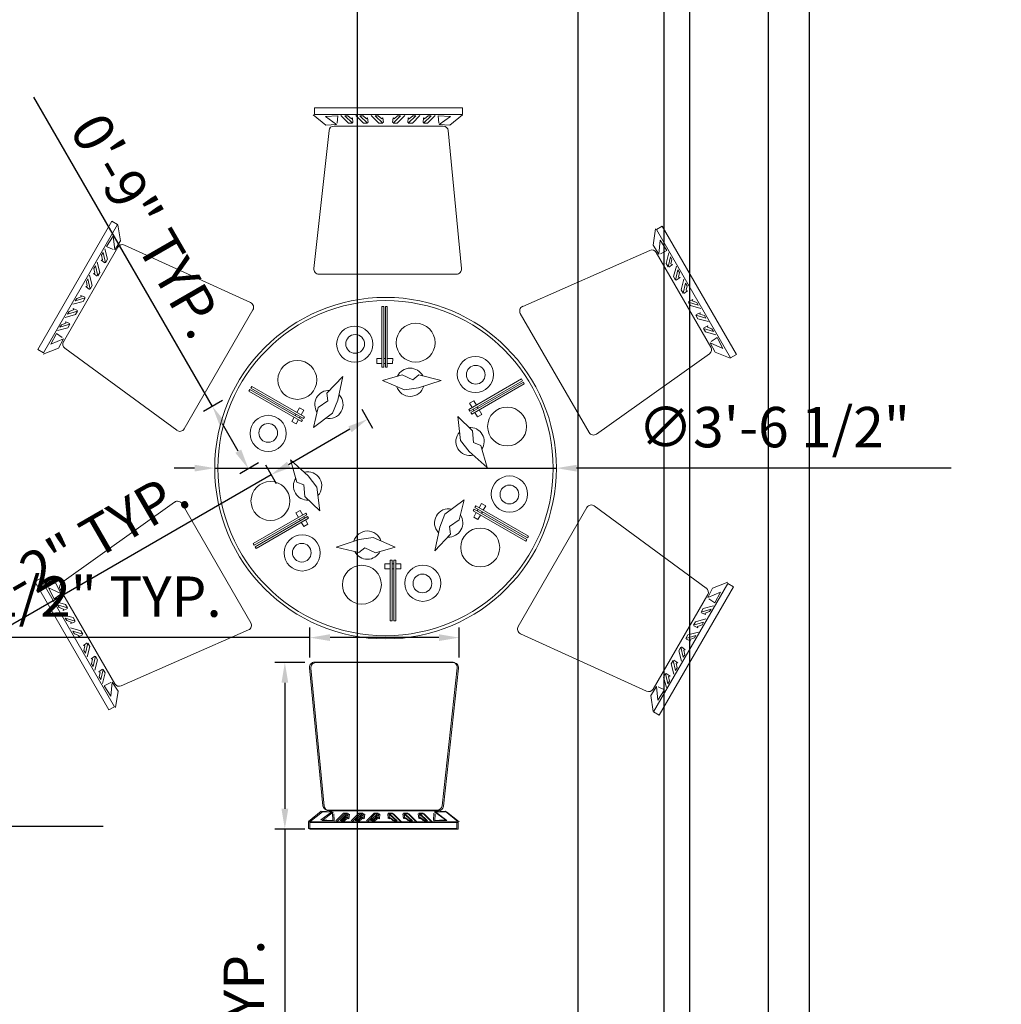
# Model space of a CAD drawing. Units: inches. Extents: x 2923 to 3500, y 1684 to 2381.
# Tile 8 of 12: x 3125 to 3246, y 1992 to 2114. Entities that reach past the tile are written whole.
import ezdxf

# ---------------------------------------------------------------- set-up
doc = ezdxf.new("R2010")
doc.units = ezdxf.units.IN
doc.layers.add('A-ANNO-DIMS', color=2, linetype='Continuous', lineweight=18)
doc.layers.add('Furniture', color=7, linetype='Continuous', lineweight=15)
doc.styles.get("Standard").update_dxf_attribs({"font": 'txt', "height": 5})
doc.dimstyles.new('ISO-25', dxfattribs={"dimtxt": 5, "dimasz": 2.5, "dimexe": 1.25, "dimexo": 0.625, "dimtad": 1, "dimlunit": 3, "dimtxsty": 'Standard', "dimcen": 2.5, "dimadec": 0, "dimazin": 0, "dimtfac": 1, "dimtmove": 0, "dimatfit": 3, "dimfxl": 1, "dimarcsym": 0})

# ---------------------------------------------------------------- blocks, each defined once
blk = doc.blocks.new('CHAIR-DINING')
for p, q in [((0, 19.73), (1.57, 18.47)), ((0.13, 20.61), (0.13, 19.79)), ((18.48, 20.61), (0.13, 20.61)), ((0.13, 19.79), (18.48, 19.79)), ((1.51, 19.54), (3.02, 19.6)), ((2.89, 18.53), (1.51, 19.54)), ((3.02, 19.6), (2.95, 18.72)), ((3.39, 19.66), (4.34, 18.72)), ((3.9, 19.6), (4.27, 19.6)), ((4.84, 18.72), (3.9, 19.6)), ((4.27, 19.6), (4.71, 19.22)), ((5.28, 19.66), (6.22, 18.72)), ((5.78, 19.6), (6.16, 19.6)), ((6.73, 18.72), (5.78, 19.6)), ((6.16, 19.6), (6.6, 19.22)), ((7.16, 19.66), (8.11, 18.72)), ((7.67, 19.6), (8.04, 19.6)), ((8.61, 18.72), (7.67, 19.6)), ((8.04, 19.6), (8.48, 19.22)), ((9.87, 18.72), (10.81, 19.6)), ((10.43, 19.6), (9.99, 19.22)), ((11.31, 19.66), (10.37, 18.72)), ((10.81, 19.6), (10.43, 19.6)), ((11.75, 18.72), (12.7, 19.6)), ((12.32, 19.6), (11.88, 19.22)), ((13.2, 19.66), (12.26, 18.72)), ((12.7, 19.6), (12.32, 19.6)), ((13.64, 18.72), (14.58, 19.6)), ((14.2, 19.6), (13.76, 19.22)), ((15.08, 19.66), (14.14, 18.72)), ((14.58, 19.6), (14.2, 19.6)), ((15.46, 19.6), (15.52, 18.72)), ((16.97, 19.54), (15.46, 19.6)), ((15.59, 18.53), (16.97, 19.54)), ((18.48, 19.73), (16.91, 18.47)), ((18.48, 19.79), (18.48, 20.61)), ((1.57, 18.47), (2.89, 18.53)), ((2.57, 18.34), (16.08, 18.34)), ((4.34, 18.72), (4.84, 18.72)), ((4.71, 19.22), (4.84, 19.35)), ((4.84, 19.35), (4.9, 18.78)), ((6.22, 18.72), (6.73, 18.72)), ((6.6, 19.22), (6.73, 19.35)), ((6.73, 19.35), (6.79, 18.78)), ((8.11, 18.72), (8.61, 18.72)), ((8.48, 19.22), (8.61, 19.35)), ((8.61, 19.35), (8.67, 18.78)), ((9.87, 19.35), (9.8, 18.78)), ((9.99, 19.22), (9.87, 19.35)), ((10.37, 18.72), (9.87, 18.72)), ((11.75, 19.35), (11.69, 18.78)), ((11.88, 19.22), (11.75, 19.35)), ((12.26, 18.72), (11.75, 18.72)), ((13.64, 19.35), (13.58, 18.78)), ((13.76, 19.22), (13.64, 19.35)), ((14.14, 18.72), (13.64, 18.72)), ((16.91, 18.47), (15.59, 18.53)), ((0.08, 0.7), (1.95, 17.78)), ((16.71, 17.78), (18.35, 0.69)), ((17.72, 0), (0.7, 0))]:
    blk.add_line(p, q)
for centre, start, end in [((2.57, 17.72), 90, 173.7428), ((16.08, 17.72), 5.4801, 90), ((0.7, 0.63), 173.7428, 270), ((17.72, 0.63), 270, 5.4801)]:
    blk.add_arc(centre, 0.629, start, end)
blk = doc.blocks.new('TABLE-PLACE-SETTING')
for p, q in [((8.13, 10.96, 3.57), (1.62, 7.2, 3.57)), ((1.74, 6.99, 3.57), (8.25, 10.75, 3.57)), ((8.35, 10.57, 3.57), (1.84, 6.81, 3.57)), ((1.96, 6.61, 3.57), (8.47, 10.37, 3.57)), ((8.25, 10.75, 3.57), (8.13, 10.96, 3.57)), ((8.47, 10.37, 3.57), (8.35, 10.57, 3.57)), ((2.23, 8.25, 3.57), (1.7, 7.95, 3.57)), ((1.7, 7.95, 3.57), (2.01, 7.42, 3.57)), ((2.54, 7.72, 3.57), (2.23, 8.25, 3.57)), ((2.76, 7.34, 3.57), (2.65, 7.52, 3.57)), ((2.07, 4.55, 3.57), (0.25, 6.3, 3.57)), ((0.25, 6.3, 3.57), (0.59, 3.36, 3.57)), ((1.62, 7.2, 3.57), (1.74, 6.99, 3.57)), ((1.84, 6.81, 3.57), (1.96, 6.61, 3.57)), ((2.12, 7.22, 3.57), (2.23, 7.03, 3.57)), ((2.35, 6.83, 3.57), (2.68, 6.26, 3.57)), ((2.68, 6.26, 3.57), (3.21, 6.56, 3.57)), ((3.21, 6.56, 3.57), (2.88, 7.13, 3.57)), ((2.19, 3.1, 3.57), (2.07, 4.55, 3.57)), ((0.59, 3.36, 3.57), (1.66, 1.99, 3.57)), ((3.08, 2.74, 3.57), (2.19, 3.1, 3.57)), ((3.88, 0, 3.57), (3.08, 2.74, 3.57)), ((1.66, 1.99, 3.57), (3.88, 0, 3.57))]:
    blk.add_line(p, q)
for centre, radius in [((2.41, 11.52, 3.57), 2.24), ((2.46, 11.49, 3.57), 1.16), ((6.34, 5.08, 3.57), 2.41)]:
    blk.add_circle(centre, radius)
for start, end in [(326.6641, 94.1442), (137.0611, 284.0662)]:
    blk.add_arc((1.75, 3.22, 3.57), 1.75, start, end)
blk = doc.blocks.new('*D37')
at = {"layer": 'A-ANNO-DIMS', "color": 0, "lineweight": -2, "transparency": 16777216}
for p, q in [((3021, 2017.25), (3021, 2012.78)), ((3046.61, 2017.25), (3046.61, 2012.78)), ((3023.5, 2014.03), (3044.11, 2014.03)), ((3046.61, 2014.03), (3134.88, 2014.03))]:
    blk.add_line(p, q, dxfattribs=at)
at = {"layer": 'A-ANNO-DIMS', "color": 0, "transparency": 16777216}
for points in [[(3023.5, 2014.45), (3023.5, 2013.61), (3021, 2014.03)], [(3044.11, 2014.45), (3044.11, 2013.61), (3046.61, 2014.03)]]:
    blk.add_solid(points, dxfattribs=at)
at = {"layer": 'Defpoints', "color": 0, "transparency": 16777216}
for p in [(3021, 2017.87), (3046.61, 2017.87), (3046.61, 2014.03)]:
    blk.add_point(p, dxfattribs=at)
at = {"layer": 'A-ANNO-DIMS', "color": 0, "transparency": 16777216, "insert": (3092, 2018.46), "char_height": 5, "attachment_point": 5}
blk.add_mtext('BASIN 2\'-1 1/2" TYP.', dxfattribs=at)
blk = doc.blocks.new('*D39')
at = {"layer": 'A-ANNO-DIMS', "color": 0, "lineweight": -2, "transparency": 16777216}
for p, q in [((3159.85, 2034.29), (3156.13, 2034.29)), ((3157.38, 2031.79), (3157.38, 2016.18)), ((3159.85, 2013.68), (3156.13, 2013.68)), ((3157.38, 2013.68), (3157.38, 1925.17))]:
    blk.add_line(p, q, dxfattribs=at)
at = {"layer": 'A-ANNO-DIMS', "color": 0, "transparency": 16777216}
for points in [[(3156.96, 2031.79), (3157.8, 2031.79), (3157.38, 2034.29)], [(3156.96, 2016.18), (3157.8, 2016.18), (3157.38, 2013.68)]]:
    blk.add_solid(points, dxfattribs=at)
at = {"layer": 'Defpoints', "color": 0, "transparency": 16777216}
for p in [(3160.47, 2034.29), (3157.38, 2013.68), (3160.47, 2013.68)]:
    blk.add_point(p, dxfattribs=at)
at = {"layer": 'A-ANNO-DIMS', "color": 0, "transparency": 16777216, "insert": (3152.94, 1968.18), "char_height": 5, "attachment_point": 5, "rotation": 90}
blk.add_mtext('CHAIR 1\'-8 1/2" TYP.', dxfattribs=at)
blk = doc.blocks.new('*D40')
at = {"layer": 'A-ANNO-DIMS', "color": 0, "lineweight": -2, "transparency": 16777216}
for p, q in [((3160.47, 2034.91), (3160.47, 2038.63)), ((3178.95, 2034.91), (3178.95, 2038.63)), ((3160.47, 2037.38), (3098.86, 2037.38)), ((3176.45, 2037.38), (3162.97, 2037.38))]:
    blk.add_line(p, q, dxfattribs=at)
at = {"layer": 'A-ANNO-DIMS', "color": 0, "transparency": 16777216}
for points in [[(3162.97, 2037.8), (3162.97, 2036.96), (3160.47, 2037.38)], [(3176.45, 2037.8), (3176.45, 2036.96), (3178.95, 2037.38)]]:
    blk.add_solid(points, dxfattribs=at)
at = {"layer": 'Defpoints', "color": 0, "transparency": 16777216}
for p in [(3160.47, 2037.38), (3160.47, 2034.29), (3178.95, 2034.29)]:
    blk.add_point(p, dxfattribs=at)
at = {"layer": 'A-ANNO-DIMS', "color": 0, "transparency": 16777216, "insert": (3128.42, 2041.81), "char_height": 5, "attachment_point": 5}
blk.add_mtext('1\'-6 1/2" TYP.', dxfattribs=at)
blk = doc.blocks.new('*D41')
at = {"layer": 'A-ANNO-DIMS', "color": 0, "lineweight": -2, "transparency": 16777216}
for p, q in [((3166.89, 2065.67), (3168.23, 2063.34)), ((3165.44, 2063.18), (3157.85, 2058.8)), ((3154.97, 2058.79), (3156.31, 2056.46)), ((3155.69, 2057.55), (3088.31, 2018.65))]:
    blk.add_line(p, q, dxfattribs=at)
at = {"layer": 'A-ANNO-DIMS', "color": 0, "transparency": 16777216}
for points in [[(3165.23, 2063.54), (3165.65, 2062.82), (3167.61, 2064.43)], [(3157.64, 2059.16), (3158.06, 2058.43), (3155.69, 2057.55)]]:
    blk.add_solid(points, dxfattribs=at)
at = {"layer": 'Defpoints', "color": 0, "transparency": 16777216}
for p in [(3166.57, 2066.21), (3154.66, 2059.33), (3155.69, 2057.55)]:
    blk.add_point(p, dxfattribs=at)
at = {"layer": 'A-ANNO-DIMS', "color": 0, "transparency": 16777216, "insert": (3119.12, 2040.59), "char_height": 5, "attachment_point": 5, "rotation": 30}
blk.add_mtext('SETTING 1\'-2" TYP.', dxfattribs=at)
blk = doc.blocks.new('*D42')
at = {"layer": 'A-ANNO-DIMS', "color": 0, "lineweight": -2, "transparency": 16777216}
for p, q in [((3148.42, 2066.01), (3126.3, 2104.31)), ((3149.66, 2066.73), (3147.33, 2065.39)), ((3151.62, 2060.47), (3149.67, 2063.85)), ((3154.11, 2059.02), (3151.79, 2057.68))]:
    blk.add_line(p, q, dxfattribs=at)
at = {"layer": 'A-ANNO-DIMS', "color": 0, "transparency": 16777216}
for points in [[(3150.03, 2064.06), (3149.31, 2063.64), (3148.42, 2066.01)], [(3151.98, 2060.67), (3151.26, 2060.26), (3152.87, 2058.3)]]:
    blk.add_solid(points, dxfattribs=at)
at = {"layer": 'Defpoints', "color": 0, "transparency": 16777216}
for p in [(3150.2, 2067.04), (3148.42, 2066.01), (3154.66, 2059.33)]:
    blk.add_point(p, dxfattribs=at)
at = {"layer": 'A-ANNO-DIMS', "color": 0, "transparency": 16777216, "insert": (3139.85, 2088.05), "char_height": 5, "attachment_point": 5, "rotation": 300}
blk.add_mtext('0\'-9" TYP.', dxfattribs=at)
blk = doc.blocks.new('*D49')
at = {"layer": 'A-ANNO-DIMS', "color": 0, "lineweight": -2, "transparency": 16777216}
for p, q in [((2969.23, 2263.03), (2969.23, 2370.16)), ((3444.23, 2110.03), (3444.23, 2370.16)), ((2971.73, 2368.91), (3441.73, 2368.91))]:
    blk.add_line(p, q, dxfattribs=at)
at = {"layer": 'A-ANNO-DIMS', "color": 0, "transparency": 16777216}
for points in [[(2971.73, 2369.32), (2971.73, 2368.49), (2969.23, 2368.91)], [(3441.73, 2369.32), (3441.73, 2368.49), (3444.23, 2368.91)]]:
    blk.add_solid(points, dxfattribs=at)
at = {"layer": 'Defpoints', "color": 0, "transparency": 16777216}
for p in [(3444.23, 2368.91), (2969.23, 2262.41), (3444.23, 2109.41)]:
    blk.add_point(p, dxfattribs=at)
at = {"layer": 'A-ANNO-DIMS', "color": 0, "transparency": 16777216, "insert": (3206.73, 2372.51), "char_height": 5, "attachment_point": 5}
blk.add_mtext('39\'-7"', dxfattribs=at)
blk = doc.blocks.new('*D54')
at = {"layer": 'A-ANNO-DIMS', "color": 0, "lineweight": -2, "transparency": 16777216}
for p, q in [((3166.32, 2236.75), (3166.32, 1685.66)), ((3193.64, 2236.75), (3193.64, 1685.66)), ((3168.82, 1686.91), (3191.14, 1686.91)), ((3193.64, 1686.91), (3235.49, 1686.91))]:
    blk.add_line(p, q, dxfattribs=at)
at = {"layer": 'A-ANNO-DIMS', "color": 0, "transparency": 16777216}
for points in [[(3168.82, 1687.32), (3168.82, 1686.49), (3166.32, 1686.91)], [(3191.14, 1687.32), (3191.14, 1686.49), (3193.64, 1686.91)]]:
    blk.add_solid(points, dxfattribs=at)
at = {"layer": 'Defpoints', "color": 0, "transparency": 16777216}
for p in [(3166.32, 2237.38), (3193.64, 2237.38), (3193.64, 1686.91)]:
    blk.add_point(p, dxfattribs=at)
at = {"layer": 'A-ANNO-DIMS', "color": 0, "transparency": 16777216, "insert": (3215.82, 1691.34), "char_height": 5, "attachment_point": 5}
blk.add_mtext('2\'-3 1/2"', dxfattribs=at)
blk = doc.blocks.new('*D62')
at = {"layer": 'A-ANNO-DIMS', "color": 0, "lineweight": -2, "transparency": 16777216}
for p, q in [((3204.33, 1920.39), (3204.33, 2370.16)), ((3217.26, 1920.39), (3217.26, 2370.16)), ((3206.83, 2368.91), (3214.76, 2368.91)), ((3217.26, 2368.91), (3238.87, 2368.91))]:
    blk.add_line(p, q, dxfattribs=at)
at = {"layer": 'A-ANNO-DIMS', "color": 0, "transparency": 16777216}
for points in [[(3206.83, 2369.32), (3206.83, 2368.49), (3204.33, 2368.91)], [(3214.76, 2369.32), (3214.76, 2368.49), (3217.26, 2368.91)]]:
    blk.add_solid(points, dxfattribs=at)
at = {"layer": 'Defpoints', "color": 0, "transparency": 16777216}
for p in [(3217.26, 2368.91), (3204.33, 1919.77), (3217.26, 1919.77)]:
    blk.add_point(p, dxfattribs=at)
at = {"layer": 'A-ANNO-DIMS', "color": 0, "transparency": 16777216, "insert": (3229.31, 2372.51), "char_height": 5, "attachment_point": 5}
blk.add_mtext('1\'-1"', dxfattribs=at)
blk = doc.blocks.new('*D66')
at = {"layer": 'A-ANNO-DIMS', "color": 0, "lineweight": -2, "transparency": 16777216}
for p, q in [((3207.52, 1946.69), (3207.52, 2370.16)), ((3222.33, 1946.69), (3222.33, 2370.16)), ((3210.02, 2368.91), (3219.83, 2368.91)), ((3222.33, 2368.91), (3244.89, 2368.91))]:
    blk.add_line(p, q, dxfattribs=at)
at = {"layer": 'A-ANNO-DIMS', "color": 0, "transparency": 16777216}
for points in [[(3210.02, 2369.32), (3210.02, 2368.49), (3207.52, 2368.91)], [(3219.83, 2369.32), (3219.83, 2368.49), (3222.33, 2368.91)]]:
    blk.add_solid(points, dxfattribs=at)
at = {"layer": 'Defpoints', "color": 0, "transparency": 16777216}
for p in [(3222.33, 2368.91), (3207.52, 1946.07), (3222.33, 1946.07)]:
    blk.add_point(p, dxfattribs=at)
at = {"layer": 'A-ANNO-DIMS', "color": 0, "transparency": 16777216, "insert": (3234.86, 2372.51), "char_height": 5, "attachment_point": 5}
blk.add_mtext('1\'-3"', dxfattribs=at)
blk = doc.blocks.new('*D72')
at = {"layer": 'A-ANNO-DIMS', "color": 0, "lineweight": -2, "transparency": 16777216}
for p, q in [((3146.2, 2058.37), (3143.7, 2058.37)), ((3148.7, 2058.37), (3190.99, 2058.37)), ((3239.86, 2058.37), (3193.49, 2058.37))]:
    blk.add_line(p, q, dxfattribs=at)
at = {"layer": 'A-ANNO-DIMS', "color": 0, "transparency": 16777216}
for points in [[(3146.2, 2058.79), (3146.2, 2057.95), (3148.7, 2058.37)], [(3193.49, 2058.78), (3193.49, 2057.95), (3190.99, 2058.37)]]:
    blk.add_solid(points, dxfattribs=at)
at = {"layer": 'Defpoints', "color": 0, "transparency": 16777216}
for p in [(3148.7, 2058.37), (3190.99, 2058.37)]:
    blk.add_point(p, dxfattribs=at)
at = {"layer": 'A-ANNO-DIMS', "color": 0, "transparency": 16777216, "insert": (3217.92, 2062.8), "char_height": 5, "attachment_point": 5, "rotation": 359.9992}
blk.add_mtext('∅3\'-6 1/2"', dxfattribs=at)

msp = doc.modelspace()

# ---------------------------------------------------------------- linework, layer by layer
at = {"layer": 'Furniture'}
for radius in [21.143, 20.749]:
    msp.add_circle((3169.843, 2058.368), radius, dxfattribs=at)

# ---------------------------------------------------------------- block references
for name, p in [('CHAIR-DINING', (3160.9, 2082.389)), ('TABLE-PLACE-SETTING', (3178.549, 2058.45))]:
    msp.add_blockref(name, p, dxfattribs=at)
for name, p, rotation in [('CHAIR-DINING', (3144.569, 2062.633), 59.99999999999123), ('CHAIR-DINING', (3186.174, 2078.124), 300.0000000000017), ('TABLE-PLACE-SETTING', (3174.803, 2065.877), 60.00000000001655), ('TABLE-PLACE-SETTING', (3166.498, 2066.346), 120.0000000000032), ('TABLE-PLACE-SETTING', (3161.94, 2059.388), 180), ('TABLE-PLACE-SETTING', (3173.99, 2051.492), 300.0000000000044), ('CHAIR-DINING', (3153.513, 2038.613), 120.0000000000018), ('CHAIR-DINING', (3195.118, 2054.103), 240.0000000000047), ('TABLE-PLACE-SETTING', (3165.686, 2051.962), 239.9999999999923), ('CHAIR-DINING', (3178.787, 2034.348), 180), ('CHAIR-DINING', (3178.949, 2034.288), 180)]:
    msp.add_blockref(name, p, dxfattribs=dict(at, rotation=rotation))

# ---------------------------------------------------------------- dimensions: what is measured, and where the dimension line sits
at = {"layer": 'A-ANNO-DIMS'}
for base, p1, p2, picture, middle in [((3444.23, 2368.906), (2969.23, 2262.406), (3444.23, 2109.406), '*D49', (3206.73, 2372.507)), ((3217.261, 2368.906), (3204.334, 1919.766), (3217.261, 1919.766), '*D62', (3229.315, 2372.507)), ((3222.331, 2368.906), (3207.519, 1946.066), (3222.331, 1946.066), '*D66', (3234.86, 2372.507)), ((3193.644, 1686.906), (3166.316, 2237.38), (3193.644, 2237.38), '*D54', (3215.817, 1691.341))]:
    dim = msp.add_linear_dim(base=base, p1=p1, p2=p2, dimstyle='ISO-25', override={"dimdec": 1, "dimlfac": 1, "dimrnd": 0, "dimzin": 1, "dimdsep": 46, "dimlunit": 4, "dimfrac": 2}, dxfattribs=at)
    dim.commit()
    dim.dimension.update_dxf_attribs({"geometry": picture, "text_midpoint": middle})
for base, p1, p2, angle, text, picture, middle in [((3148.417, 2066.012), (3154.656, 2059.333), (3150.204, 2067.044), 120, '<> TYP.', '*D42', (3139.854, 2088.045)), ((3155.688, 2057.545), (3166.574, 2066.214), (3154.656, 2059.333), 210, 'SETTING <> TYP.', '*D41', (3119.118, 2040.59)), ((3160.47, 2037.379), (3178.949, 2034.288), (3160.47, 2034.288), 180, '<> TYP.', '*D40', (3128.417, 2041.814)), ((3157.38, 2013.683), (3160.47, 2034.288), (3160.47, 2013.683), 270, 'CHAIR <> TYP.', '*D39', (3152.945, 1968.177))]:
    dim = msp.add_linear_dim(base=base, p1=p1, p2=p2, angle=angle, text=text, dimstyle='ISO-25', override={"dimdec": 1, "dimlfac": 1, "dimrnd": 0, "dimzin": 1, "dimdsep": 46, "dimlunit": 4, "dimfrac": 2}, dxfattribs=at)
    dim.commit()
    dim.dimension.update_dxf_attribs({"geometry": picture, "text_midpoint": middle})
dim = msp.add_diameter_dim_2p(p1=(3148.701, 2058.369), p2=(3190.986, 2058.368), dimstyle='ISO-25', override={"dimdec": 1, "dimlfac": 1, "dimrnd": 0, "dimzin": 1, "dimdsep": 46, "dimlunit": 4, "dimfrac": 2}, dxfattribs=at)
dim.commit()
dim.dimension.update_dxf_attribs({"geometry": '*D72', "text_midpoint": (3217.921, 2058.368), "dimtype": 163})
dim = msp.add_linear_dim(base=(3046.609, 2014.029), p1=(3020.997, 2017.871), p2=(3046.609, 2017.871), text='BASIN <> TYP.', dimstyle='ISO-25', override={"dimdec": 1, "dimlfac": 1, "dimrnd": 0, "dimzin": 1, "dimdsep": 46, "dimlunit": 4, "dimfrac": 2}, dxfattribs=at)
dim.commit()
dim.dimension.update_dxf_attribs({"geometry": '*D37', "text_midpoint": (3091.996, 2018.464)})

doc.saveas('drawing.dxf')
